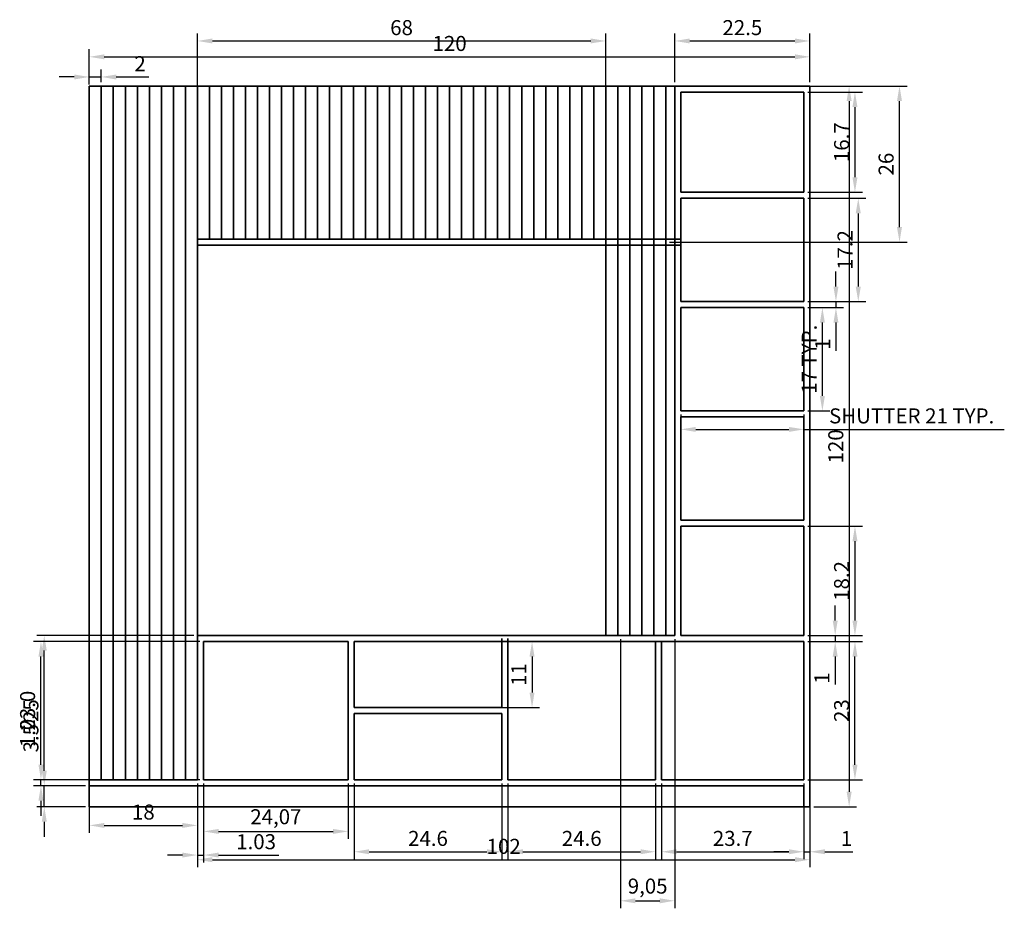
# Model space of a CAD drawing. Units: inches. Extents: x 50 to 214, y 31 to 179.
import ezdxf

# ---------------------------------------------------------------- set-up
doc = ezdxf.new("R2010")
doc.units = ezdxf.units.IN
doc.layers.add('A-ANNO-DIMS', color=2, linetype='Continuous', lineweight=18)
doc.layers.add('A-FURN', color=7, linetype='Continuous', lineweight=35)
doc.styles.get("Standard").update_dxf_attribs({"font": 'arial.ttf'})
doc.dimstyles.new('ISO-25', dxfattribs={"dimtxt": 2.5, "dimasz": 2.5, "dimexe": 1.25, "dimexo": 0.625, "dimtad": 1, "dimtxsty": 'Standard', "dimcen": 2.5, "dimadec": 0, "dimazin": 0, "dimtfac": 1, "dimtmove": 0, "dimatfit": 3, "dimfxl": 1, "dimarcsym": 0})

# ---------------------------------------------------------------- blocks, each defined once
blk = doc.blocks.new('*D1')
at = {"layer": 'A-ANNO-DIMS', "color": 0, "lineweight": -2, "transparency": 16777216}
for p, q in [((61.97, 167.74), (61.97, 173.58)), ((64.47, 172.33), (179.47, 172.33)), ((181.97, 168.1), (181.97, 173.58))]:
    blk.add_line(p, q, dxfattribs=at)
at = {"layer": 'A-ANNO-DIMS', "color": 0, "transparency": 16777216}
for points in [[(64.47, 172.75), (64.47, 171.91), (61.97, 172.33)], [(179.47, 172.75), (179.47, 171.91), (181.97, 172.33)]]:
    blk.add_solid(points, dxfattribs=at)
at = {"layer": 'Defpoints', "color": 0, "transparency": 16777216}
for p in [(181.97, 172.33), (181.97, 167.47), (61.97, 167.11)]:
    blk.add_point(p, dxfattribs=at)
at = {"layer": 'A-ANNO-DIMS', "color": 0, "transparency": 16777216, "insert": (121.97, 174.23), "char_height": 2.5, "attachment_point": 5}
blk.add_mtext('120', dxfattribs=at)
blk = doc.blocks.new('*D2')
at = {"layer": 'A-ANNO-DIMS', "color": 0, "lineweight": -2, "transparency": 16777216}
for p, q in [((182.6, 167.47), (189.75, 167.47)), ((188.5, 164.97), (188.5, 49.97)), ((182.6, 47.47), (189.75, 47.47))]:
    blk.add_line(p, q, dxfattribs=at)
at = {"layer": 'A-ANNO-DIMS', "color": 0, "transparency": 16777216}
for points in [[(188.08, 164.97), (188.92, 164.97), (188.5, 167.47)], [(188.08, 49.97), (188.92, 49.97), (188.5, 47.47)]]:
    blk.add_solid(points, dxfattribs=at)
at = {"layer": 'Defpoints', "color": 0, "transparency": 16777216}
for p in [(181.97, 167.47), (181.97, 47.47), (188.5, 47.47)]:
    blk.add_point(p, dxfattribs=at)
at = {"layer": 'A-ANNO-DIMS', "color": 0, "transparency": 16777216, "insert": (186.6, 107.47), "char_height": 2.5, "attachment_point": 5, "rotation": 90}
blk.add_mtext('120', dxfattribs=at)
blk = doc.blocks.new('*D3')
at = {"layer": 'A-ANNO-DIMS', "color": 0, "lineweight": -2, "transparency": 16777216}
for p, q in [((186.3, 134.07), (186.3, 136.57)), ((181.6, 131.57), (187.55, 131.57)), ((186.3, 131.57), (186.3, 130.57)), ((181.6, 130.57), (187.55, 130.57)), ((186.3, 128.07), (186.3, 123.4))]:
    blk.add_line(p, q, dxfattribs=at)
at = {"layer": 'A-ANNO-DIMS', "color": 0, "transparency": 16777216}
for points in [[(185.89, 134.07), (186.72, 134.07), (186.3, 131.57)], [(185.89, 128.07), (186.72, 128.07), (186.3, 130.57)]]:
    blk.add_solid(points, dxfattribs=at)
at = {"layer": 'Defpoints', "color": 0, "transparency": 16777216}
for p in [(180.97, 131.57), (180.97, 130.57), (186.3, 130.57)]:
    blk.add_point(p, dxfattribs=at)
at = {"layer": 'A-ANNO-DIMS', "color": 0, "transparency": 16777216, "insert": (184.42, 124.49), "char_height": 2.5, "attachment_point": 5, "rotation": 90}
blk.add_mtext('1', dxfattribs=at)
blk = doc.blocks.new('*D4')
at = {"layer": 'A-ANNO-DIMS', "color": 0, "lineweight": -2, "transparency": 16777216}
for p, q in [((186.18, 78.47), (186.18, 80.97)), ((181.6, 75.97), (187.43, 75.97)), ((186.18, 75.97), (186.18, 74.97)), ((181.6, 74.97), (187.43, 74.97)), ((186.18, 72.47), (186.18, 67.8))]:
    blk.add_line(p, q, dxfattribs=at)
at = {"layer": 'A-ANNO-DIMS', "color": 0, "transparency": 16777216}
for points in [[(185.76, 78.47), (186.6, 78.47), (186.18, 75.97)], [(185.76, 72.47), (186.6, 72.47), (186.18, 74.97)]]:
    blk.add_solid(points, dxfattribs=at)
at = {"layer": 'Defpoints', "color": 0, "transparency": 16777216}
for p in [(180.97, 75.97), (180.97, 74.97), (186.18, 74.97)]:
    blk.add_point(p, dxfattribs=at)
at = {"layer": 'A-ANNO-DIMS', "color": 0, "transparency": 16777216, "insert": (184.3, 68.89), "char_height": 2.5, "attachment_point": 5, "rotation": 90}
blk.add_mtext('1', dxfattribs=at)
blk = doc.blocks.new('*D5')
at = {"layer": 'A-ANNO-DIMS', "color": 0, "lineweight": -2, "transparency": 16777216}
for p, q in [((59.47, 168.98), (56.97, 168.98)), ((61.97, 168.1), (61.97, 170.23)), ((61.97, 168.98), (63.97, 168.98)), ((63.97, 168.1), (63.97, 170.23)), ((66.47, 168.98), (71.88, 168.98))]:
    blk.add_line(p, q, dxfattribs=at)
at = {"layer": 'A-ANNO-DIMS', "color": 0, "transparency": 16777216}
for points in [[(59.47, 169.39), (59.47, 168.56), (61.97, 168.98)], [(66.47, 169.39), (66.47, 168.56), (63.97, 168.98)]]:
    blk.add_solid(points, dxfattribs=at)
at = {"layer": 'Defpoints', "color": 0, "transparency": 16777216}
for p in [(63.97, 168.98), (61.97, 167.47), (63.97, 167.47)]:
    blk.add_point(p, dxfattribs=at)
at = {"layer": 'A-ANNO-DIMS', "color": 0, "transparency": 16777216, "insert": (70.42, 170.86), "char_height": 2.5, "attachment_point": 5}
blk.add_mtext('2', dxfattribs=at)
blk = doc.blocks.new('*D6')
at = {"layer": 'A-ANNO-DIMS', "color": 0, "lineweight": -2, "transparency": 16777216}
for p, q in [((61.97, 51.35), (61.97, 43.11)), ((79.97, 51.35), (79.97, 43.11)), ((64.47, 44.36), (77.47, 44.36))]:
    blk.add_line(p, q, dxfattribs=at)
at = {"layer": 'A-ANNO-DIMS', "color": 0, "transparency": 16777216}
for points in [[(64.47, 44.77), (64.47, 43.94), (61.97, 44.36)], [(77.47, 44.77), (77.47, 43.94), (79.97, 44.36)]]:
    blk.add_solid(points, dxfattribs=at)
at = {"layer": 'Defpoints', "color": 0, "transparency": 16777216}
for p in [(61.97, 51.97), (79.97, 51.97), (79.97, 44.36)]:
    blk.add_point(p, dxfattribs=at)
at = {"layer": 'A-ANNO-DIMS', "color": 0, "transparency": 16777216, "insert": (70.97, 46.26), "char_height": 2.5, "attachment_point": 5}
blk.add_mtext('18', dxfattribs=at)
blk = doc.blocks.new('*D7')
at = {"layer": 'A-ANNO-DIMS', "color": 0, "lineweight": -2, "transparency": 16777216}
for p, q in [((79.97, 51.35), (79.97, 37.4)), ((181.97, 51.35), (181.97, 37.4)), ((82.47, 38.65), (179.47, 38.65))]:
    blk.add_line(p, q, dxfattribs=at)
at = {"layer": 'A-ANNO-DIMS', "color": 0, "transparency": 16777216}
for points in [[(82.47, 39.07), (82.47, 38.23), (79.97, 38.65)], [(179.47, 39.07), (179.47, 38.23), (181.97, 38.65)]]:
    blk.add_solid(points, dxfattribs=at)
at = {"layer": 'Defpoints', "color": 0, "transparency": 16777216}
for p in [(79.97, 51.97), (181.97, 51.97), (181.97, 38.65)]:
    blk.add_point(p, dxfattribs=at)
at = {"layer": 'A-ANNO-DIMS', "color": 0, "transparency": 16777216, "insert": (130.97, 40.55), "char_height": 2.5, "attachment_point": 5}
blk.add_mtext('102', dxfattribs=at)
blk = doc.blocks.new('*D8')
at = {"layer": 'A-ANNO-DIMS', "color": 0, "lineweight": -2, "transparency": 16777216}
for p, q in [((81, 51.35), (81, 42.11)), ((105.07, 51.35), (105.07, 42.11)), ((83.5, 43.36), (102.57, 43.36))]:
    blk.add_line(p, q, dxfattribs=at)
at = {"layer": 'A-ANNO-DIMS', "color": 0, "transparency": 16777216}
for points in [[(83.5, 43.77), (83.5, 42.94), (81, 43.36)], [(102.57, 43.77), (102.57, 42.94), (105.07, 43.36)]]:
    blk.add_solid(points, dxfattribs=at)
at = {"layer": 'Defpoints', "color": 0, "transparency": 16777216}
for p in [(81, 51.97), (105.07, 51.97), (105.07, 43.36)]:
    blk.add_point(p, dxfattribs=at)
at = {"layer": 'A-ANNO-DIMS', "color": 0, "transparency": 16777216, "insert": (93.04, 45.48), "char_height": 2.5, "attachment_point": 5}
blk.add_mtext('24,07', dxfattribs=at)
blk = doc.blocks.new('*D9')
at = {"layer": 'A-ANNO-DIMS', "color": 0, "lineweight": -2, "transparency": 16777216}
for p, q in [((106.7, 74.97), (136.95, 74.97)), ((135.7, 72.47), (135.7, 66.47)), ((106.7, 63.97), (136.95, 63.97))]:
    blk.add_line(p, q, dxfattribs=at)
at = {"layer": 'A-ANNO-DIMS', "color": 0, "transparency": 16777216}
for points in [[(135.28, 72.47), (136.11, 72.47), (135.7, 74.97)], [(135.28, 66.47), (136.11, 66.47), (135.7, 63.97)]]:
    blk.add_solid(points, dxfattribs=at)
at = {"layer": 'Defpoints', "color": 0, "transparency": 16777216}
for p in [(106.07, 74.97), (106.07, 63.97), (135.7, 63.97)]:
    blk.add_point(p, dxfattribs=at)
at = {"layer": 'A-ANNO-DIMS', "color": 0, "transparency": 16777216, "insert": (133.82, 69.47), "char_height": 2.5, "attachment_point": 5, "rotation": 90}
blk.add_mtext('11', dxfattribs=at)
blk = doc.blocks.new('*D10')
at = {"layer": 'A-ANNO-DIMS', "color": 0, "lineweight": -2, "transparency": 16777216}
for p, q in [((158.6, 167.47), (198.14, 167.47)), ((196.89, 143.97), (196.89, 164.97)), ((158.6, 141.47), (198.14, 141.47))]:
    blk.add_line(p, q, dxfattribs=at)
at = {"layer": 'A-ANNO-DIMS', "color": 0, "transparency": 16777216}
for points in [[(196.47, 164.97), (197.3, 164.97), (196.89, 167.47)], [(196.47, 143.97), (197.3, 143.97), (196.89, 141.47)]]:
    blk.add_solid(points, dxfattribs=at)
at = {"layer": 'Defpoints', "color": 0, "transparency": 16777216}
for p in [(157.97, 167.47), (196.89, 167.47), (157.97, 141.47)]:
    blk.add_point(p, dxfattribs=at)
at = {"layer": 'A-ANNO-DIMS', "color": 0, "transparency": 16777216, "insert": (194.98, 154.47), "char_height": 2.5, "attachment_point": 5, "rotation": 90}
blk.add_mtext('26', dxfattribs=at)
blk = doc.blocks.new('*D11')
at = {"layer": 'A-ANNO-DIMS', "color": 0, "lineweight": -2, "transparency": 16777216}
for p, q in [((150.42, 75.35), (150.42, 30.56)), ((159.47, 75.35), (159.47, 30.56)), ((152.92, 31.81), (156.97, 31.81))]:
    blk.add_line(p, q, dxfattribs=at)
at = {"layer": 'A-ANNO-DIMS', "color": 0, "transparency": 16777216}
for points in [[(152.92, 32.22), (152.92, 31.39), (150.42, 31.81)], [(156.97, 32.22), (156.97, 31.39), (159.47, 31.81)]]:
    blk.add_solid(points, dxfattribs=at)
at = {"layer": 'Defpoints', "color": 0, "transparency": 16777216}
for p in [(150.42, 75.97), (159.47, 75.97), (159.47, 31.81)]:
    blk.add_point(p, dxfattribs=at)
at = {"layer": 'A-ANNO-DIMS', "color": 0, "transparency": 16777216, "insert": (154.95, 33.93), "char_height": 2.5, "attachment_point": 5}
blk.add_mtext('9,05', dxfattribs=at)
blk = doc.blocks.new('SHUTTER-PANEL')
for p, q in [((0, 17.2), (20.5, 17.2)), ((0, 0), (0, 17.2)), ((20.5, 0), (20.5, 17.2)), ((0, 0), (20.5, 0))]:
    blk.add_line(p, q)
blk = doc.blocks.new('*D13')
at = {"layer": 'A-ANNO-DIMS', "color": 0, "lineweight": -2, "transparency": 16777216}
for p, q in [((160.47, 112.75), (160.47, 109.05)), ((180.97, 112.75), (180.97, 109.05)), ((162.97, 110.3), (178.47, 110.3)), ((180.97, 110.3), (214.34, 110.3))]:
    blk.add_line(p, q, dxfattribs=at)
at = {"layer": 'A-ANNO-DIMS', "color": 0, "transparency": 16777216}
for points in [[(162.97, 110.71), (162.97, 109.88), (160.47, 110.3)], [(178.47, 110.71), (178.47, 109.88), (180.97, 110.3)]]:
    blk.add_solid(points, dxfattribs=at)
at = {"layer": 'Defpoints', "color": 0, "transparency": 16777216}
for p in [(160.47, 113.37), (180.97, 113.37), (180.97, 110.3)]:
    blk.add_point(p, dxfattribs=at)
at = {"layer": 'A-ANNO-DIMS', "color": 0, "transparency": 16777216, "insert": (198.91, 112.22), "char_height": 2.5, "attachment_point": 5}
blk.add_mtext('SHUTTER 21 TYP.', dxfattribs=at)
blk = doc.blocks.new('*D14')
at = {"layer": 'A-ANNO-DIMS', "color": 0, "lineweight": -2, "transparency": 16777216}
for p, q in [((181.6, 130.57), (185.3, 130.57)), ((184.05, 115.87), (184.05, 128.07)), ((181.6, 113.37), (185.3, 113.37))]:
    blk.add_line(p, q, dxfattribs=at)
at = {"layer": 'A-ANNO-DIMS', "color": 0, "transparency": 16777216}
for points in [[(183.63, 128.07), (184.46, 128.07), (184.05, 130.57)], [(183.63, 115.87), (184.46, 115.87), (184.05, 113.37)]]:
    blk.add_solid(points, dxfattribs=at)
at = {"layer": 'Defpoints', "color": 0, "transparency": 16777216}
for p in [(180.97, 130.57), (184.05, 130.57), (180.97, 113.37)]:
    blk.add_point(p, dxfattribs=at)
at = {"layer": 'A-ANNO-DIMS', "color": 0, "transparency": 16777216, "insert": (182.17, 121.97), "char_height": 2.5, "attachment_point": 5, "rotation": 90}
blk.add_mtext('17 TYP.', dxfattribs=at)
blk = doc.blocks.new('*D15')
at = {"layer": 'A-ANNO-DIMS', "color": 0, "lineweight": -2, "transparency": 16777216}
for p, q in [((54.47, 53.47), (54.47, 61.79)), ((61.35, 50.97), (53.22, 50.97)), ((54.47, 47.47), (54.47, 50.97)), ((61.35, 47.47), (53.22, 47.47)), ((54.47, 44.97), (54.47, 42.47))]:
    blk.add_line(p, q, dxfattribs=at)
at = {"layer": 'A-ANNO-DIMS', "color": 0, "transparency": 16777216}
for points in [[(54.05, 53.47), (54.89, 53.47), (54.47, 50.97)], [(54.05, 44.97), (54.89, 44.97), (54.47, 47.47)]]:
    blk.add_solid(points, dxfattribs=at)
at = {"layer": 'Defpoints', "color": 0, "transparency": 16777216}
for p in [(54.47, 50.97), (61.97, 50.97), (61.97, 47.47)]:
    blk.add_point(p, dxfattribs=at)
at = {"layer": 'A-ANNO-DIMS', "color": 0, "transparency": 16777216, "insert": (52.57, 58.88), "char_height": 2.5, "attachment_point": 5, "rotation": 90}
blk.add_mtext('3.5', dxfattribs=at)
blk = doc.blocks.new('*D16')
at = {"layer": 'A-ANNO-DIMS', "color": 0, "lineweight": -2, "transparency": 16777216}
for p, q in [((181.6, 74.97), (190.72, 74.97)), ((189.47, 54.47), (189.47, 72.47)), ((181.6, 51.97), (190.72, 51.97))]:
    blk.add_line(p, q, dxfattribs=at)
at = {"layer": 'A-ANNO-DIMS', "color": 0, "transparency": 16777216}
for points in [[(189.05, 72.47), (189.89, 72.47), (189.47, 74.97)], [(189.05, 54.47), (189.89, 54.47), (189.47, 51.97)]]:
    blk.add_solid(points, dxfattribs=at)
at = {"layer": 'Defpoints', "color": 0, "transparency": 16777216}
for p in [(180.97, 74.97), (189.47, 74.97), (180.97, 51.97)]:
    blk.add_point(p, dxfattribs=at)
at = {"layer": 'A-ANNO-DIMS', "color": 0, "transparency": 16777216, "insert": (187.57, 63.47), "char_height": 2.5, "attachment_point": 5, "rotation": 90}
blk.add_mtext('23', dxfattribs=at)
blk = doc.blocks.new('*D17')
at = {"layer": 'A-ANNO-DIMS', "color": 0, "lineweight": -2, "transparency": 16777216}
for p, q in [((79.35, 75.97), (53.22, 75.97)), ((54.47, 53.47), (54.47, 73.47)), ((61.35, 50.97), (53.22, 50.97))]:
    blk.add_line(p, q, dxfattribs=at)
at = {"layer": 'A-ANNO-DIMS', "color": 0, "transparency": 16777216}
for points in [[(54.05, 73.47), (54.89, 73.47), (54.47, 75.97)], [(54.05, 53.47), (54.89, 53.47), (54.47, 50.97)]]:
    blk.add_solid(points, dxfattribs=at)
at = {"layer": 'Defpoints', "color": 0, "transparency": 16777216}
for p in [(54.47, 75.97), (79.97, 75.97), (61.97, 50.97)]:
    blk.add_point(p, dxfattribs=at)
at = {"layer": 'A-ANNO-DIMS', "color": 0, "transparency": 16777216, "insert": (52.57, 63.47), "char_height": 2.5, "attachment_point": 5, "rotation": 90}
blk.add_mtext('25', dxfattribs=at)
blk = doc.blocks.new('*D18')
at = {"layer": 'A-ANNO-DIMS', "color": 0, "lineweight": -2, "transparency": 16777216}
for p, q in [((180.97, 50.35), (180.97, 38.72)), ((181.97, 46.85), (181.97, 38.72)), ((178.47, 39.97), (175.97, 39.97)), ((180.97, 39.97), (181.97, 39.97)), ((184.47, 39.97), (189.14, 39.97))]:
    blk.add_line(p, q, dxfattribs=at)
at = {"layer": 'A-ANNO-DIMS', "color": 0, "transparency": 16777216}
for points in [[(178.47, 40.39), (178.47, 39.56), (180.97, 39.97)], [(184.47, 40.39), (184.47, 39.56), (181.97, 39.97)]]:
    blk.add_solid(points, dxfattribs=at)
at = {"layer": 'Defpoints', "color": 0, "transparency": 16777216}
for p in [(180.97, 50.97), (181.97, 47.47), (181.97, 39.97)]:
    blk.add_point(p, dxfattribs=at)
at = {"layer": 'A-ANNO-DIMS', "color": 0, "transparency": 16777216, "insert": (188.06, 41.85), "char_height": 2.5, "attachment_point": 5}
blk.add_mtext('1', dxfattribs=at)
blk = doc.blocks.new('*D19')
at = {"layer": 'A-ANNO-DIMS', "color": 0, "lineweight": -2, "transparency": 16777216}
for p, q in [((106.07, 51.35), (106.07, 38.72)), ((130.67, 51.35), (130.67, 38.72)), ((108.57, 39.97), (128.17, 39.97))]:
    blk.add_line(p, q, dxfattribs=at)
at = {"layer": 'A-ANNO-DIMS', "color": 0, "transparency": 16777216}
for points in [[(108.57, 40.39), (108.57, 39.56), (106.07, 39.97)], [(128.17, 40.39), (128.17, 39.56), (130.67, 39.97)]]:
    blk.add_solid(points, dxfattribs=at)
at = {"layer": 'Defpoints', "color": 0, "transparency": 16777216}
for p in [(106.07, 51.97), (130.67, 51.97), (130.67, 39.97)]:
    blk.add_point(p, dxfattribs=at)
at = {"layer": 'A-ANNO-DIMS', "color": 0, "transparency": 16777216, "insert": (118.37, 41.87), "char_height": 2.5, "attachment_point": 5}
blk.add_mtext('24.6', dxfattribs=at)
blk = doc.blocks.new('*D20')
at = {"layer": 'A-ANNO-DIMS', "color": 0, "lineweight": -2, "transparency": 16777216}
for p, q in [((131.67, 51.35), (131.67, 38.72)), ((156.27, 51.35), (156.27, 38.72)), ((134.17, 39.97), (153.77, 39.97))]:
    blk.add_line(p, q, dxfattribs=at)
at = {"layer": 'A-ANNO-DIMS', "color": 0, "transparency": 16777216}
for points in [[(134.17, 40.39), (134.17, 39.56), (131.67, 39.97)], [(153.77, 40.39), (153.77, 39.56), (156.27, 39.97)]]:
    blk.add_solid(points, dxfattribs=at)
at = {"layer": 'Defpoints', "color": 0, "transparency": 16777216}
for p in [(131.67, 51.97), (156.27, 51.97), (156.27, 39.97)]:
    blk.add_point(p, dxfattribs=at)
at = {"layer": 'A-ANNO-DIMS', "color": 0, "transparency": 16777216, "insert": (143.97, 41.87), "char_height": 2.5, "attachment_point": 5}
blk.add_mtext('24.6', dxfattribs=at)
blk = doc.blocks.new('*D21')
at = {"layer": 'A-ANNO-DIMS', "color": 0, "lineweight": -2, "transparency": 16777216}
for p, q in [((157.27, 51.35), (157.27, 38.72)), ((180.97, 51.35), (180.97, 38.72)), ((159.77, 39.97), (178.47, 39.97))]:
    blk.add_line(p, q, dxfattribs=at)
at = {"layer": 'A-ANNO-DIMS', "color": 0, "transparency": 16777216}
for points in [[(159.77, 40.39), (159.77, 39.56), (157.27, 39.97)], [(178.47, 40.39), (178.47, 39.56), (180.97, 39.97)]]:
    blk.add_solid(points, dxfattribs=at)
at = {"layer": 'Defpoints', "color": 0, "transparency": 16777216}
for p in [(157.27, 51.97), (180.97, 51.97), (180.97, 39.97)]:
    blk.add_point(p, dxfattribs=at)
at = {"layer": 'A-ANNO-DIMS', "color": 0, "transparency": 16777216, "insert": (169.12, 41.87), "char_height": 2.5, "attachment_point": 5}
blk.add_mtext('23.7', dxfattribs=at)
blk = doc.blocks.new('*D22')
at = {"layer": 'A-ANNO-DIMS', "color": 0, "lineweight": -2, "transparency": 16777216}
for p, q in [((159.47, 168.1), (159.47, 176.22)), ((181.97, 168.1), (181.97, 176.22)), ((161.97, 174.97), (179.47, 174.97))]:
    blk.add_line(p, q, dxfattribs=at)
at = {"layer": 'A-ANNO-DIMS', "color": 0, "transparency": 16777216}
for points in [[(161.97, 175.39), (161.97, 174.56), (159.47, 174.97)], [(179.47, 175.39), (179.47, 174.56), (181.97, 174.97)]]:
    blk.add_solid(points, dxfattribs=at)
at = {"layer": 'Defpoints', "color": 0, "transparency": 16777216}
for p in [(181.97, 174.97), (159.47, 167.47), (181.97, 167.47)]:
    blk.add_point(p, dxfattribs=at)
at = {"layer": 'A-ANNO-DIMS', "color": 0, "transparency": 16777216, "insert": (170.72, 176.87), "char_height": 2.5, "attachment_point": 5}
blk.add_mtext('22.5', dxfattribs=at)
blk = doc.blocks.new('*D23')
at = {"layer": 'A-ANNO-DIMS', "color": 0, "lineweight": -2, "transparency": 16777216}
for p, q in [((181.6, 166.47), (190.72, 166.47)), ((189.47, 163.97), (189.47, 152.27)), ((181.6, 149.77), (190.72, 149.77))]:
    blk.add_line(p, q, dxfattribs=at)
at = {"layer": 'A-ANNO-DIMS', "color": 0, "transparency": 16777216}
for points in [[(189.05, 163.97), (189.89, 163.97), (189.47, 166.47)], [(189.05, 152.27), (189.89, 152.27), (189.47, 149.77)]]:
    blk.add_solid(points, dxfattribs=at)
at = {"layer": 'Defpoints', "color": 0, "transparency": 16777216}
for p in [(180.97, 166.47), (180.97, 149.77), (189.47, 149.77)]:
    blk.add_point(p, dxfattribs=at)
at = {"layer": 'A-ANNO-DIMS', "color": 0, "transparency": 16777216, "insert": (187.57, 158.12), "char_height": 2.5, "attachment_point": 5, "rotation": 90}
blk.add_mtext('16.7', dxfattribs=at)
blk = doc.blocks.new('*D24')
at = {"layer": 'A-ANNO-DIMS', "color": 0, "lineweight": -2, "transparency": 16777216}
for p, q in [((181.6, 94.17), (190.72, 94.17)), ((189.47, 91.67), (189.47, 78.47)), ((181.6, 75.97), (190.72, 75.97))]:
    blk.add_line(p, q, dxfattribs=at)
at = {"layer": 'A-ANNO-DIMS', "color": 0, "transparency": 16777216}
for points in [[(189.05, 91.67), (189.89, 91.67), (189.47, 94.17)], [(189.05, 78.47), (189.89, 78.47), (189.47, 75.97)]]:
    blk.add_solid(points, dxfattribs=at)
at = {"layer": 'Defpoints', "color": 0, "transparency": 16777216}
for p in [(180.97, 94.17), (180.97, 75.97), (189.47, 75.97)]:
    blk.add_point(p, dxfattribs=at)
at = {"layer": 'A-ANNO-DIMS', "color": 0, "transparency": 16777216, "insert": (187.57, 85.07), "char_height": 2.5, "attachment_point": 5, "rotation": 90}
blk.add_mtext('18.2', dxfattribs=at)
blk = doc.blocks.new('*D25')
at = {"layer": 'A-ANNO-DIMS', "color": 0, "lineweight": -2, "transparency": 16777216}
for p, q in [((79.97, 141.6), (79.97, 176.22)), ((147.97, 142.1), (147.97, 176.22)), ((82.47, 174.97), (145.47, 174.97))]:
    blk.add_line(p, q, dxfattribs=at)
at = {"layer": 'A-ANNO-DIMS', "color": 0, "transparency": 16777216}
for points in [[(82.47, 175.39), (82.47, 174.56), (79.97, 174.97)], [(145.47, 175.39), (145.47, 174.56), (147.97, 174.97)]]:
    blk.add_solid(points, dxfattribs=at)
at = {"layer": 'Defpoints', "color": 0, "transparency": 16777216}
for p in [(147.97, 174.97), (147.97, 141.47), (79.97, 140.97)]:
    blk.add_point(p, dxfattribs=at)
at = {"layer": 'A-ANNO-DIMS', "color": 0, "transparency": 16777216, "insert": (113.97, 176.87), "char_height": 2.5, "attachment_point": 5}
blk.add_mtext('68', dxfattribs=at)
blk = doc.blocks.new('*D26')
at = {"layer": 'A-ANNO-DIMS', "color": 0, "lineweight": -2, "transparency": 16777216}
for p, q in [((181.6, 148.77), (191.27, 148.77)), ((190.02, 146.27), (190.02, 134.07)), ((181.6, 131.57), (191.27, 131.57))]:
    blk.add_line(p, q, dxfattribs=at)
at = {"layer": 'A-ANNO-DIMS', "color": 0, "transparency": 16777216}
for points in [[(189.6, 146.27), (190.44, 146.27), (190.02, 148.77)], [(189.6, 134.07), (190.44, 134.07), (190.02, 131.57)]]:
    blk.add_solid(points, dxfattribs=at)
at = {"layer": 'Defpoints', "color": 0, "transparency": 16777216}
for p in [(180.97, 148.77), (180.97, 131.57), (190.02, 131.57)]:
    blk.add_point(p, dxfattribs=at)
at = {"layer": 'A-ANNO-DIMS', "color": 0, "transparency": 16777216, "insert": (188.14, 140.17), "char_height": 2.5, "attachment_point": 5, "rotation": 90}
blk.add_mtext('17.2', dxfattribs=at)
blk = doc.blocks.new('*D27')
at = {"layer": 'A-ANNO-DIMS', "color": 0, "lineweight": -2, "transparency": 16777216}
for p, q in [((80.37, 74.97), (52.67, 74.97)), ((53.92, 54.47), (53.92, 72.47)), ((80.37, 51.97), (52.67, 51.97))]:
    blk.add_line(p, q, dxfattribs=at)
at = {"layer": 'A-ANNO-DIMS', "color": 0, "transparency": 16777216}
for points in [[(53.5, 72.47), (54.34, 72.47), (53.92, 74.97)], [(53.5, 54.47), (54.34, 54.47), (53.92, 51.97)]]:
    blk.add_solid(points, dxfattribs=at)
at = {"layer": 'Defpoints', "color": 0, "transparency": 16777216}
for p in [(53.92, 74.97), (81, 74.97), (81, 51.97)]:
    blk.add_point(p, dxfattribs=at)
at = {"layer": 'A-ANNO-DIMS', "color": 0, "transparency": 16777216, "insert": (52.02, 63.47), "char_height": 2.5, "attachment_point": 5, "rotation": 90}
blk.add_mtext('23.0', dxfattribs=at)
blk = doc.blocks.new('*D28')
at = {"layer": 'A-ANNO-DIMS', "color": 0, "lineweight": -2, "transparency": 16777216}
for p, q in [((53.92, 54.47), (53.92, 62.53)), ((61.35, 51.97), (52.67, 51.97)), ((61.35, 50.97), (52.67, 50.97)), ((53.92, 50.97), (53.92, 51.97)), ((53.92, 48.47), (53.92, 45.97))]:
    blk.add_line(p, q, dxfattribs=at)
at = {"layer": 'A-ANNO-DIMS', "color": 0, "transparency": 16777216}
for points in [[(53.5, 54.47), (54.34, 54.47), (53.92, 51.97)], [(53.5, 48.47), (54.34, 48.47), (53.92, 50.97)]]:
    blk.add_solid(points, dxfattribs=at)
at = {"layer": 'Defpoints', "color": 0, "transparency": 16777216}
for p in [(53.92, 51.97), (61.97, 51.97), (61.97, 50.97)]:
    blk.add_point(p, dxfattribs=at)
at = {"layer": 'A-ANNO-DIMS', "color": 0, "transparency": 16777216, "insert": (52.02, 59.75), "char_height": 2.5, "attachment_point": 5, "rotation": 90}
blk.add_mtext('1.0', dxfattribs=at)
blk = doc.blocks.new('*D29')
at = {"layer": 'A-ANNO-DIMS', "color": 0, "lineweight": -2, "transparency": 16777216}
for p, q in [((79.97, 51.35), (79.97, 38.17)), ((81, 51.35), (81, 38.17)), ((77.47, 39.42), (74.97, 39.42)), ((79.97, 39.42), (81, 39.42)), ((83.5, 39.42), (93.51, 39.42))]:
    blk.add_line(p, q, dxfattribs=at)
at = {"layer": 'A-ANNO-DIMS', "color": 0, "transparency": 16777216}
for points in [[(77.47, 39.84), (77.47, 39.01), (79.97, 39.42)], [(83.5, 39.84), (83.5, 39.01), (81, 39.42)]]:
    blk.add_solid(points, dxfattribs=at)
at = {"layer": 'Defpoints', "color": 0, "transparency": 16777216}
for p in [(79.97, 51.97), (81, 51.97), (81, 39.42)]:
    blk.add_point(p, dxfattribs=at)
at = {"layer": 'A-ANNO-DIMS', "color": 0, "transparency": 16777216, "insert": (89.75, 41.32), "char_height": 2.5, "attachment_point": 5}
blk.add_mtext('1.03', dxfattribs=at)

msp = doc.modelspace()

# ---------------------------------------------------------------- linework, layer by layer
at = {"layer": 'A-FURN'}
for p, q in [((181.971, 167.472), (61.971, 167.472)), ((61.971, 167.472), (61.971, 47.472)), ((63.971, 167.472), (63.971, 141.472)), ((65.971, 167.472), (65.971, 141.472)), ((65.971, 167.472), (65.971, 141.472)), ((67.971, 167.472), (67.971, 141.472)), ((67.971, 167.472), (67.971, 141.472)), ((69.971, 167.472), (69.971, 141.472)), ((69.971, 167.472), (69.971, 141.472)), ((71.971, 167.472), (71.971, 141.472)), ((71.971, 167.472), (71.971, 141.472)), ((73.971, 167.472), (73.971, 141.472)), ((73.971, 167.472), (73.971, 141.472)), ((75.971, 167.472), (75.971, 141.472)), ((75.971, 167.472), (75.971, 141.472)), ((77.971, 167.472), (77.971, 141.472)), ((77.971, 167.472), (77.971, 141.472)), ((79.971, 167.472), (79.971, 141.472)), ((79.971, 167.472), (79.971, 141.472)), ((81.971, 167.472), (81.971, 141.972)), ((81.971, 167.472), (81.971, 141.972)), ((83.971, 167.472), (83.971, 141.972)), ((83.971, 167.472), (83.971, 141.972)), ((85.971, 167.472), (85.971, 141.972)), ((85.971, 167.472), (85.971, 141.972)), ((87.971, 167.472), (87.971, 141.972)), ((87.971, 167.472), (87.971, 141.972)), ((87.971, 167.472), (87.971, 141.972)), ((89.971, 167.472), (89.971, 141.972)), ((89.971, 167.472), (89.971, 141.972)), ((89.971, 167.472), (89.971, 141.972)), ((91.971, 167.472), (91.971, 141.972)), ((91.971, 167.472), (91.971, 141.972)), ((91.971, 167.472), (91.971, 141.972)), ((93.971, 167.472), (93.971, 141.972)), ((93.971, 167.472), (93.971, 141.972)), ((93.971, 167.472), (93.971, 141.972)), ((95.971, 167.472), (95.971, 141.972)), ((95.971, 167.472), (95.971, 141.972)), ((95.971, 167.472), (95.971, 141.972)), ((97.971, 167.472), (97.971, 141.972)), ((97.971, 167.472), (97.971, 141.972)), ((97.971, 167.472), (97.971, 141.972)), ((99.971, 167.472), (99.971, 141.972)), ((99.971, 167.472), (99.971, 141.972)), ((99.971, 167.472), (99.971, 141.972)), ((99.971, 167.472), (99.971, 141.972)), ((101.971, 167.472), (101.971, 141.972)), ((101.971, 167.472), (101.971, 141.972)), ((101.971, 167.472), (101.971, 141.972)), ((103.971, 167.472), (103.971, 141.972)), ((103.971, 167.472), (103.971, 141.972)), ((105.971, 167.472), (105.971, 141.972)), ((105.971, 167.472), (105.971, 141.972)), ((107.971, 167.472), (107.971, 141.972)), ((107.971, 167.472), (107.971, 141.972)), ((109.971, 167.472), (109.971, 141.972)), ((111.971, 167.472), (111.971, 141.972)), ((113.971, 167.472), (113.971, 141.972)), ((115.971, 167.472), (115.971, 141.972)), ((117.971, 167.472), (117.971, 141.972)), ((119.971, 167.472), (119.971, 141.972)), ((119.971, 167.472), (119.971, 141.972)), ((121.971, 167.472), (121.971, 141.972)), ((123.971, 167.472), (123.971, 141.972)), ((125.971, 167.472), (125.971, 141.972)), ((127.971, 167.472), (127.971, 141.972)), ((129.971, 167.472), (129.971, 141.972)), ((131.971, 167.472), (131.971, 141.972)), ((133.971, 167.472), (133.971, 141.972)), ((135.971, 167.472), (135.971, 141.972)), ((137.971, 167.472), (137.971, 141.972)), ((139.971, 167.472), (139.971, 141.972)), ((141.971, 167.472), (141.971, 141.972)), ((143.971, 167.472), (143.971, 141.972)), ((145.971, 167.472), (145.971, 141.972)), ((147.971, 167.472), (147.971, 141.472)), ((149.971, 167.472), (149.971, 141.472)), ((149.971, 75.972), (149.971, 167.472)), ((151.971, 167.472), (151.971, 141.472)), ((151.971, 75.972), (151.971, 167.472)), ((153.971, 167.472), (153.971, 141.472)), ((153.971, 75.972), (153.971, 167.472)), ((155.971, 167.472), (155.971, 141.472)), ((155.971, 75.972), (155.971, 167.472)), ((157.971, 167.472), (157.971, 141.472)), ((157.971, 75.972), (157.971, 167.472)), ((159.471, 75.972), (159.471, 167.472)), ((159.971, 167.472), (181.971, 167.472)), ((181.971, 47.472), (181.971, 167.472)), ((160.471, 166.472), (180.971, 166.472)), ((160.471, 149.772), (160.471, 166.472)), ((180.971, 149.772), (180.971, 166.472)), ((160.471, 149.772), (180.971, 149.772)), ((63.971, 141.472), (63.971, 51.972)), ((65.971, 141.472), (65.971, 51.972)), ((65.971, 141.472), (65.971, 75.472)), ((67.971, 141.472), (67.971, 51.972)), ((67.971, 141.472), (67.971, 75.472)), ((69.971, 141.472), (69.971, 51.972)), ((69.971, 141.472), (69.971, 75.472)), ((71.971, 141.472), (71.971, 51.972)), ((71.971, 141.472), (71.971, 75.472)), ((73.971, 141.472), (73.971, 51.972)), ((73.971, 141.472), (73.971, 75.472)), ((75.971, 141.472), (75.971, 51.972)), ((75.971, 141.472), (75.971, 75.472)), ((77.971, 141.472), (77.971, 51.972)), ((77.971, 141.472), (77.971, 75.472)), ((79.971, 141.972), (160.471, 141.972)), ((79.971, 141.472), (79.971, 51.972)), ((79.971, 141.472), (79.971, 75.472)), ((147.971, 141.472), (147.971, 75.972)), ((149.971, 141.472), (149.971, 75.972)), ((151.971, 141.472), (151.971, 75.972)), ((153.971, 141.472), (153.971, 75.972)), ((155.971, 141.472), (155.971, 75.972)), ((157.971, 141.472), (157.971, 75.972)), ((79.971, 140.972), (160.471, 140.972)), ((160.471, 94.172), (180.971, 94.172)), ((160.471, 75.972), (160.471, 94.172)), ((180.971, 75.972), (180.971, 94.172)), ((65.971, 75.472), (65.971, 51.972)), ((67.971, 75.472), (67.971, 51.972)), ((69.971, 75.472), (69.971, 51.972)), ((71.971, 75.472), (71.971, 51.972)), ((73.971, 75.472), (73.971, 51.972)), ((75.971, 75.472), (75.971, 51.972)), ((77.971, 75.472), (77.971, 51.972)), ((79.971, 75.972), (149.425, 75.972)), ((79.971, 75.472), (79.971, 51.972)), ((130.671, 75.472), (130.671, 63.972)), ((131.671, 75.472), (131.671, 51.972)), ((149.425, 75.972), (159.471, 75.972)), ((160.471, 75.972), (180.971, 75.972)), ((80.999, 74.972), (105.071, 74.972)), ((80.999, 74.972), (80.999, 51.972)), ((105.071, 74.972), (105.071, 51.972)), ((106.071, 74.972), (106.071, 63.972)), ((106.071, 74.972), (180.971, 74.972)), ((156.271, 74.972), (156.271, 51.972)), ((157.271, 74.972), (157.271, 51.972)), ((180.971, 51.972), (180.971, 74.972)), ((106.071, 63.972), (130.671, 63.972)), ((106.071, 62.972), (130.671, 62.972)), ((106.071, 62.972), (106.071, 51.972)), ((130.671, 62.972), (130.671, 51.972)), ((61.971, 51.972), (79.971, 51.972)), ((61.971, 50.972), (180.971, 50.972)), ((80.999, 51.972), (105.071, 51.972)), ((106.071, 51.972), (130.671, 51.972)), ((131.671, 51.972), (156.271, 51.972)), ((157.271, 51.972), (180.971, 51.972)), ((180.971, 47.472), (180.971, 50.972)), ((61.971, 47.472), (181.971, 47.472))]:
    msp.add_line(p, q, dxfattribs=at)

# ---------------------------------------------------------------- block references
at = {"layer": 'A-FURN', "rotation": 180}
msp.add_blockref('SHUTTER-PANEL', (180.972, 148.773), dxfattribs=at)
at = {"layer": 'A-FURN'}
for p in [(160.471, 113.372), (160.471, 95.172)]:
    msp.add_blockref('SHUTTER-PANEL', p, dxfattribs=at)

# ---------------------------------------------------------------- dimensions: what is measured, and where the dimension line sits
at = {"layer": 'A-ANNO-DIMS'}
for base, p1, p2, override, picture, middle in [((147.971, 174.972), (79.971, 140.972), (147.971, 141.472), {"dimdec": 0, "dimlfac": 1, "dimrnd": 0, "dimzin": 0, "dimdsep": 46, "dimlunit": 2}, '*D25', (113.971, 176.874)), ((181.971, 174.972), (159.471, 167.472), (181.971, 167.472), {"dimdec": 1, "dimlfac": 1, "dimrnd": 0, "dimzin": 0, "dimdsep": 46, "dimlunit": 2}, '*D22', (170.721, 176.874)), ((181.971, 172.33), (61.971, 167.114), (181.971, 167.472), {"dimclrd": 0, "dimclre": 0, "dimclrt": 0}, '*D1', (121.971, 174.232)), ((63.971, 168.978), (61.971, 167.472), (63.971, 167.472), {"dimclrd": 0, "dimclre": 0, "dimclrt": 0}, '*D5', (70.424, 170.858)), ((159.471, 31.805), (150.425, 75.972), (159.471, 75.972), {"dimclrd": 0, "dimclre": 0, "dimclrt": 0}, '*D11', (154.948, 33.933)), ((79.971, 44.356), (61.971, 51.972), (79.971, 51.972), {"dimclrd": 0, "dimclre": 0, "dimclrt": 0}, '*D6', (70.971, 46.257)), ((80.999, 39.422), (79.971, 51.972), (80.999, 51.972), {"dimdec": 2, "dimlfac": 1, "dimrnd": 0, "dimzin": 0, "dimdsep": 46, "dimlunit": 2}, '*D29', (89.753, 41.325)), ((181.971, 38.649), (79.971, 51.972), (181.971, 51.972), {"dimclrd": 0, "dimclre": 0, "dimclrt": 0}, '*D7', (130.971, 40.551)), ((105.071, 43.356), (80.999, 51.972), (105.071, 51.972), {"dimclrd": 0, "dimclre": 0, "dimclrt": 0}, '*D8', (93.035, 45.483)), ((130.671, 39.972), (106.071, 51.972), (130.671, 51.972), {"dimdec": 1, "dimlfac": 1, "dimrnd": 0, "dimzin": 0, "dimdsep": 46, "dimlunit": 2}, '*D19', (118.371, 41.874)), ((156.271, 39.972), (131.671, 51.972), (156.271, 51.972), {"dimdec": 1, "dimlfac": 1, "dimrnd": 0, "dimzin": 0, "dimdsep": 46, "dimlunit": 2}, '*D20', (143.971, 41.874)), ((180.971, 39.972), (157.271, 51.972), (180.971, 51.972), {"dimdec": 1, "dimlfac": 1, "dimrnd": 0, "dimzin": 0, "dimdsep": 46, "dimlunit": 2}, '*D21', (169.121, 41.875)), ((181.971, 39.972), (180.971, 50.972), (181.971, 47.472), {"dimdec": 0, "dimlfac": 1, "dimrnd": 0, "dimzin": 0, "dimdsep": 46, "dimlunit": 2}, '*D18', (188.057, 41.853))]:
    dim = msp.add_linear_dim(base=base, p1=p1, p2=p2, dimstyle='ISO-25', override=override, dxfattribs=at)
    dim.commit()
    dim.dimension.update_dxf_attribs({"geometry": picture, "text_midpoint": middle})
for base, p1, p2, override, picture, middle in [((196.886, 167.472), (157.971, 141.472), (157.971, 167.472), {"dimclrd": 0, "dimclre": 0, "dimclrt": 0}, '*D10', (194.984, 154.472)), ((188.499, 47.472), (181.971, 167.472), (181.971, 47.472), {"dimclrd": 0, "dimclre": 0, "dimclrt": 0}, '*D2', (186.598, 107.472)), ((189.471, 149.772), (180.971, 166.472), (180.971, 149.772), {"dimdec": 1, "dimlfac": 1, "dimrnd": 0, "dimzin": 0, "dimdsep": 46, "dimlunit": 2}, '*D23', (187.57, 158.122)), ((190.021, 131.572), (180.971, 148.772), (180.971, 131.572), {"dimdec": 1, "dimlfac": 1, "dimrnd": 0, "dimzin": 0, "dimdsep": 46, "dimlunit": 2}, '*D26', (188.141, 140.172)), ((186.302, 130.572), (180.971, 131.572), (180.971, 130.572), {"dimclrd": 0, "dimclre": 0, "dimclrt": 0}, '*D3', (184.422, 124.487)), ((189.471, 75.972), (180.971, 94.172), (180.971, 75.972), {"dimdec": 1, "dimlfac": 1, "dimrnd": 0, "dimzin": 0, "dimdsep": 46, "dimlunit": 2}, '*D24', (187.57, 85.072)), ((186.18, 74.972), (180.971, 75.972), (180.971, 74.972), {"dimclrd": 0, "dimclre": 0, "dimclrt": 0}, '*D4', (184.3, 68.887)), ((54.471, 75.972), (61.971, 50.972), (79.971, 75.972), {"dimdec": 0, "dimlfac": 1, "dimrnd": 0, "dimzin": 0, "dimdsep": 46, "dimlunit": 2}, '*D17', (52.57, 63.472)), ((53.921, 74.972), (80.999, 51.972), (80.999, 74.972), {"dimdec": 1, "dimlfac": 1, "dimrnd": 0, "dimzin": 0, "dimdsep": 46, "dimlunit": 2}, '*D27', (52.019, 63.472)), ((135.698, 63.972), (106.071, 74.972), (106.071, 63.972), {"dimclrd": 0, "dimclre": 0, "dimclrt": 0}, '*D9', (133.817, 69.472)), ((189.471, 74.972), (180.971, 51.972), (180.971, 74.972), {"dimdec": 0, "dimlfac": 1, "dimrnd": 0, "dimzin": 0, "dimdsep": 46, "dimlunit": 2}, '*D16', (187.569, 63.472)), ((53.921, 51.972), (61.971, 50.972), (61.971, 51.972), {"dimdec": 1, "dimlfac": 1, "dimrnd": 0, "dimzin": 0, "dimdsep": 46, "dimlunit": 2}, '*D28', (52.02, 59.751)), ((54.471, 50.972), (61.971, 47.472), (61.971, 50.972), {"dimdec": 1, "dimlfac": 1, "dimrnd": 0, "dimzin": 0, "dimdsep": 46, "dimlunit": 2}, '*D15', (52.569, 58.882))]:
    dim = msp.add_linear_dim(base=base, p1=p1, p2=p2, angle=90, dimstyle='ISO-25', override=override, dxfattribs=at)
    dim.commit()
    dim.dimension.update_dxf_attribs({"geometry": picture, "text_midpoint": middle})
dim = msp.add_linear_dim(base=(184.046, 130.572), p1=(180.971, 113.372), p2=(180.971, 130.572), angle=90, text='<> TYP.', dimstyle='ISO-25', override={"dimdec": 0, "dimrnd": 0, "dimzin": 0, "dimlunit": 2}, dxfattribs=at)
dim.commit()
dim.dimension.update_dxf_attribs({"geometry": '*D14', "text_midpoint": (182.165, 121.972)})
dim = msp.add_linear_dim(base=(180.97129496, 110.297467709), p1=(160.47129496, 113.372467709), p2=(180.97129496, 113.372467709), text='SHUTTER <> TYP.', dimstyle='ISO-25', override={"dimdec": 0, "dimrnd": 0, "dimzin": 0, "dimlunit": 2}, dxfattribs=at)
dim.commit()
dim.dimension.update_dxf_attribs({"geometry": '*D13', "text_midpoint": (198.906151713, 112.215100724)})

doc.saveas('drawing.dxf')
